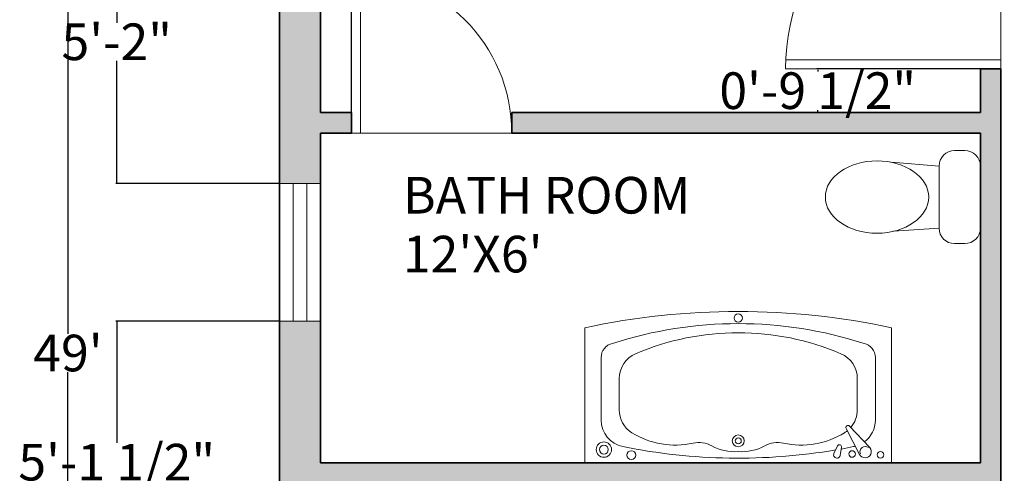
# Model space of a CAD drawing. Units: inches. Extents: x 638 to 1303, y 1 to 699.
# Tile 5 of 21: x 641 to 855, y 310 to 409. Entities that reach past the tile are written whole.
import ezdxf

# ---------------------------------------------------------------- set-up
doc = ezdxf.new("R2010")
doc.units = ezdxf.units.IN
doc.header["$MEASUREMENT"] = 0
for name, color, linetype, lineweight in [('A-ANNO-DIMS', 2, 'Continuous', 18), ('A-AREA-IDEN', 7, 'Continuous', 18), ('A-DOOR', 4, 'Continuous', 18), ('A-FLOR-FIXT', 9, 'Continuous', 18), ('A-GLAZ', 4, 'Continuous', 18), ('A-WALL', 7, 'Continuous', 35)]:
    doc.layers.add(name, color=color, linetype=linetype, lineweight=lineweight)
doc.layers.add('A-WALL-PATT', color=143, linetype='Continuous', lineweight=13, true_color=0x7aafdf)
doc.styles.get("Standard").update_dxf_attribs({"font": 'arial.ttf'})
doc.dimstyles.get("Standard").update_dxf_attribs({"dimtxt": 8, "dimasz": 0.18, "dimexe": 0.18, "dimexo": 0.0625, "dimgap": 0.09, "dimtad": 0, "dimtih": 1, "dimtoh": 1, "dimdec": 4, "dimzin": 0, "dimdsep": 46, "dimlunit": 3, "dimtxsty": 'Standard', "dimcen": 0.09, "dimadec": 0, "dimazin": 0, "dimtfac": 1, "dimtdec": 4, "dimtofl": 0, "dimtmove": 0, "dimatfit": 3, "dimfxl": 1, "dimtolj": 1, "dimtzin": 0, "dimarcsym": 0})

# ---------------------------------------------------------------- blocks, each defined once
blk = doc.blocks.new('*D1')
at = {"layer": 'A-ANNO-DIMS', "color": 0, "lineweight": -2, "transparency": 16777216}
for p, q in [((697.18, 629.82), (650.92, 629.82)), ((651.1, 629.64), (651.1, 339.99)), ((651.1, 42), (651.1, 331.64)), ((697.18, 41.82), (650.92, 41.82))]:
    blk.add_line(p, q, dxfattribs=at)
at = {"layer": 'A-ANNO-DIMS', "color": 0, "transparency": 16777216}
for points in [[(651.07, 629.64), (651.13, 629.64), (651.1, 629.82)], [(651.07, 42), (651.13, 42), (651.1, 41.82)]]:
    blk.add_solid(points, dxfattribs=at)
at = {"layer": 'Defpoints', "color": 0, "transparency": 16777216}
for p in [(697.24, 629.82), (651.1, 41.82), (697.24, 41.82)]:
    blk.add_point(p, dxfattribs=at)
at = {"layer": 'A-ANNO-DIMS', "color": 0, "transparency": 16777216, "insert": (651.1, 335.82), "char_height": 8, "attachment_point": 5}
blk.add_mtext("\\A1;49'", dxfattribs=at)
blk = doc.blocks.new('DOOR-SWING-35')
for p, q in [((33, 0), (33, 34.94)), ((35, 0), (35, 35)), ((0, 0), (35, 0))]:
    blk.add_line(p, q)
blk.add_arc((35, 0), 35, 90, 180)
blk = doc.blocks.new('WIN-30')
for p, q in [((30, 9), (0, 9)), ((0, 9), (0, 0)), ((30, 0), (30, 9)), ((0, 6), (30, 6)), ((0, 3), (30, 3)), ((0, 0), (30, 0))]:
    blk.add_line(p, q)
blk = doc.blocks.new('WC-CLOSE-COUPLED')
for p, q in [((28.2, 20.3), (30.45, 20.3)), ((24.81, 16.92), (14.41, 17.74)), ((24.81, 3.38), (24.81, 16.92)), ((33.84, 16.92), (33.84, 3.38)), ((24.81, 3.38), (14.9, 2.67)), ((30.45, 0), (28.2, 0))]:
    blk.add_line(p, q)
for centre, start, end in [((28.2, 16.92), 90, 180), ((30.45, 16.92), 0, 90), ((28.2, 3.38), 180, 270), ((30.45, 3.38), 270, 0)]:
    blk.add_arc(centre, 3.38, start, end)
blk.add_ellipse((11.28, 10.15), major_axis=(-11.28, 0), ratio=0.7)
blk = doc.blocks.new('*D57')
at = {"layer": 'A-ANNO-DIMS', "color": 0, "lineweight": -2, "transparency": 16777216}
for p, q in [((697.18, 342.79), (661.56, 342.79)), ((661.74, 342.61), (661.74, 316.23)), ((661.74, 281.4), (661.74, 307.78)), ((697.18, 281.22), (661.56, 281.22))]:
    blk.add_line(p, q, dxfattribs=at)
at = {"layer": 'A-ANNO-DIMS', "color": 0, "transparency": 16777216}
for points in [[(661.71, 342.61), (661.77, 342.61), (661.74, 342.79)], [(661.71, 281.4), (661.77, 281.4), (661.74, 281.22)]]:
    blk.add_solid(points, dxfattribs=at)
at = {"layer": 'Defpoints', "color": 0, "transparency": 16777216}
for p in [(661.74, 342.79), (697.24, 342.79), (697.24, 281.22)]:
    blk.add_point(p, dxfattribs=at)
at = {"layer": 'A-ANNO-DIMS', "color": 0, "transparency": 16777216, "insert": (661.74, 312), "char_height": 8, "attachment_point": 5}
blk.add_mtext('\\A1;5\'-1 1/2"', dxfattribs=at)
blk = doc.blocks.new('*D58')
at = {"layer": 'A-ANNO-DIMS', "color": 0, "lineweight": -2, "transparency": 16777216}
for p, q in [((697.18, 434.7), (661.56, 434.7)), ((661.74, 434.52), (661.74, 407.92)), ((661.74, 372.97), (661.74, 399.57)), ((697.18, 372.79), (661.56, 372.79))]:
    blk.add_line(p, q, dxfattribs=at)
at = {"layer": 'A-ANNO-DIMS', "color": 0, "transparency": 16777216}
for points in [[(661.71, 434.52), (661.77, 434.52), (661.74, 434.7)], [(661.71, 372.97), (661.77, 372.97), (661.74, 372.79)]]:
    blk.add_solid(points, dxfattribs=at)
at = {"layer": 'Defpoints', "color": 0, "transparency": 16777216}
for p in [(661.74, 434.7), (697.24, 434.7), (697.24, 372.79)]:
    blk.add_point(p, dxfattribs=at)
at = {"layer": 'A-ANNO-DIMS', "color": 0, "transparency": 16777216, "insert": (661.74, 403.75), "char_height": 8, "attachment_point": 5}
blk.add_mtext('\\A1;5\'-2"', dxfattribs=at)
blk = doc.blocks.new('*D66')
at = {"layer": 'A-ANNO-DIMS', "color": 0, "lineweight": -2, "transparency": 16777216}
for p, q in [((850.18, 397.83), (814.56, 397.83)), ((814.74, 397.65), (814.74, 397.3)), ((850.18, 388.32), (814.56, 388.32)), ((814.74, 388.5), (814.74, 388.85))]:
    blk.add_line(p, q, dxfattribs=at)
at = {"layer": 'A-ANNO-DIMS', "color": 0, "transparency": 16777216}
for points in [[(814.71, 397.65), (814.77, 397.65), (814.74, 397.83)], [(814.71, 388.5), (814.77, 388.5), (814.74, 388.32)]]:
    blk.add_solid(points, dxfattribs=at)
at = {"layer": 'Defpoints', "color": 0, "transparency": 16777216}
for p in [(814.74, 397.83), (850.24, 397.83), (850.24, 388.32)]:
    blk.add_point(p, dxfattribs=at)
at = {"layer": 'A-ANNO-DIMS', "color": 0, "transparency": 16777216, "insert": (814.74, 393.08), "char_height": 8, "attachment_point": 5}
blk.add_mtext('\\A1;0\'-9 1/2"', dxfattribs=at)
blk = doc.blocks.new('*D70')
at = {"layer": 'A-ANNO-DIMS', "color": 0, "lineweight": -2, "transparency": 16777216}
for p, q in [((706.24, 388.38), (706.24, 424)), ((706.42, 423.82), (712.77, 423.82)), ((712.95, 388.38), (712.95, 424)), ((712.95, 423.82), (713.13, 423.82))]:
    blk.add_line(p, q, dxfattribs=at)
at = {"layer": 'A-ANNO-DIMS', "color": 0, "transparency": 16777216}
for points in [[(706.42, 423.85), (706.42, 423.79), (706.24, 423.82)], [(712.77, 423.85), (712.77, 423.79), (712.95, 423.82)]]:
    blk.add_solid(points, dxfattribs=at)
at = {"layer": 'Defpoints', "color": 0, "transparency": 16777216}
for p in [(712.95, 423.82), (706.24, 388.32), (712.95, 388.32)]:
    blk.add_point(p, dxfattribs=at)
at = {"layer": 'A-ANNO-DIMS', "color": 0, "transparency": 16777216, "insert": (733.18, 423.82), "char_height": 8, "attachment_point": 5}
blk.add_mtext('\\A1;0\'-6 1/2"', dxfattribs=at)

msp = doc.modelspace()

# ---------------------------------------------------------------- hatches: boundary and pattern name
at = {"layer": 'A-WALL-PATT'}
h = msp.add_hatch(color=256, dxfattribs=at)
h.dxf.hatch_style = 1
h.paths.add_polyline_path([(973.34524, 629.81895), (793.35541, 629.81895), (793.35541, 620.81895), (850.23798, 620.81895), (922.23798, 620.81895), (922.23798, 524.81895), (908.94335, 524.81895), (908.94335, 520.31895), (926.73798, 520.31895), (926.73798, 544.31895), (979.3571, 544.31895), (979.3571, 548.81895), (926.73798, 548.81895), (926.73798, 620.81895), (973.34524, 620.81895)])
h.paths.add_polyline_path([(758.35541, 629.81895), (697.23798, 629.81895), (697.23798, 586.77451), (706.23798, 586.77451), (706.23798, 620.81895), (758.35541, 620.81895)])
h.paths.add_polyline_path([(1075.85281, 629.81895), (1003.34524, 629.81895), (1003.34524, 620.81895), (1046.73798, 620.81895), (1046.73798, 560.81895), (1046.73798, 548.81895), (1026.3571, 548.81895), (1026.3571, 544.31895), (1046.73798, 544.31895), (1046.73798, 486.87457), (1051.23798, 486.87457), (1051.23798, 556.31895), (1162.89753, 556.31895), (1162.89753, 560.81895), (1051.23798, 560.81895), (1051.23798, 620.81895), (1075.85281, 620.81895)])
h.paths.add_polyline_path([(1228.23798, 629.81895), (1105.85281, 629.81895), (1105.85281, 620.81895), (1219.23798, 620.81895), (1219.23798, 560.81895), (1197.89753, 560.81895), (1197.89753, 556.31895), (1219.23798, 556.31895), (1219.23798, 498.80084), (1228.23798, 498.80084)])
h.paths.add_polyline_path([(1051.23798, 439.87457), (1046.73798, 439.87457), (1046.73798, 407.81895), (1219.23798, 407.81895), (1219.23798, 381.66175), (1228.23798, 381.66175), (1228.23798, 451.80084), (1219.23798, 451.80084), (1219.23798, 412.31895), (1051.23798, 412.31895)])
h.paths.add_polyline_path([(1228.23798, 346.66175), (1219.23798, 346.66175), (1219.23798, 335.81895), (1046.73798, 335.81895), (1046.73798, 273.56895), (1051.23798, 273.56895), (1051.23798, 331.31895), (1219.23798, 331.31895), (1219.23798, 308.99654), (1228.23798, 308.99654)])
h.paths.add_polyline_path([(1228.23798, 261.99654), (1219.23798, 261.99654), (1219.23798, 211.31895), (1051.23798, 211.31895), (1051.23798, 226.56895), (1046.73798, 226.56895), (1046.73798, 211.31895), (983.84714, 211.31895), (983.84714, 206.81895), (1219.23798, 206.81895), (1219.23798, 166.83987), (1228.23798, 166.83987)])
h.paths.add_polyline_path([(1228.23798, 119.83987), (1219.23798, 119.83987), (1219.23798, 50.81895), (1197.89277, 50.81895), (1197.89277, 41.81895), (1228.23798, 41.81895)])
h.paths.add_polyline_path([(1162.89277, 50.81895), (1069.02949, 50.81895), (1069.02949, 41.81895), (1162.89277, 41.81895)])
h.paths.add_polyline_path([(1010.02949, 50.81895), (941.89631, 50.81895), (917.77455, 50.81895), (917.77455, 41.81895), (941.89631, 41.81895), (1010.02949, 41.81895)])
h.paths.add_polyline_path([(882.77455, 50.81895), (854.73798, 50.81895), (854.73798, 145.50379), (850.23798, 145.50379), (850.23798, 50.81895), (793.49755, 50.81895), (793.49755, 41.81895), (882.77455, 41.81895)])
h.paths.add_polyline_path([(746.49755, 50.81895), (706.23798, 50.81895), (706.23798, 96.57416), (697.23798, 96.57416), (697.23798, 41.81895), (746.49755, 41.81895)])
h.paths.add_polyline_path([(706.23798, 206.81895), (714.01165, 206.81895), (714.01165, 211.31895), (706.23798, 211.31895), (706.23798, 251.21966), (697.23798, 251.21966), (697.23798, 143.57416), (706.23798, 143.57416)])
h.paths.add_polyline_path([(923.84714, 211.31895), (854.73798, 211.31895), (854.73798, 397.8313), (850.23798, 397.8313), (850.23798, 388.31895), (747.9539, 388.31895), (747.9539, 383.81895), (850.23798, 383.81895), (850.23798, 311.81895), (706.23798, 311.81895), (706.23798, 342.78787), (697.23798, 342.78787), (697.23798, 281.21966), (706.23798, 281.21966), (706.23798, 307.31895), (850.23798, 307.31895), (850.23798, 211.31895), (749.01165, 211.31895), (749.01165, 206.81895), (850.23798, 206.81895), (850.23798, 192.50379), (854.73798, 192.50379), (854.73798, 206.81895), (923.84714, 206.81895)])
h.paths.add_polyline_path([(706.23798, 434.70471), (697.23798, 434.70471), (697.23798, 372.78787), (706.23798, 372.78787), (706.23798, 383.81895), (712.9539, 383.81895), (712.9539, 388.31895), (706.23798, 388.31895)])
h.paths.add_polyline_path([(706.23798, 520.31895), (850.23798, 520.31895), (850.23798, 444.8313), (854.73798, 444.8313), (854.73798, 520.31895), (861.94335, 520.31895), (861.94335, 524.81895), (706.23798, 524.81895), (706.23798, 551.77451), (697.23798, 551.77451), (697.23798, 481.70471), (706.23798, 481.70471)])

# ---------------------------------------------------------------- linework, layer by layer
at = {"layer": 'A-DOOR'}
for p, q in [((854.73798, 444.8313), (854.73798, 397.8313)), ((854.73798, 399.8313), (807.73798, 399.8313)), ((854.73798, 397.8313), (807.73798, 397.8313))]:
    msp.add_line(p, q, dxfattribs=at)
msp.add_arc((854.73798, 397.8313), 47, 90, 180, dxfattribs=at)
at = {"layer": 'A-FLOR-FIXT'}
for p, q in [((763.92818, 311.81895), (763.92818, 341.34645)), ((830.85718, 311.81895), (830.85718, 341.34645)), ((767.47148, 324.93057), (767.47148, 334.84331)), ((827.31388, 334.84331), (827.31388, 324.93057)), ((771.40848, 323.43888), (771.40848, 330.24465)), ((823.37688, 330.24465), (823.37688, 323.43888)), ((767.47148, 321.17536), (767.47148, 324.93057)), ((827.31388, 324.93057), (827.31388, 321.17536)), ((820.92178, 319.32097), (823.88637, 313.69568)), ((826.13748, 315.16947), (821.68251, 319.86636)), ((819.0491, 315.53177), (818.2862, 313.91052)), ((819.63657, 313.42497), (819.94253, 315.25261)), ((830.85718, 311.81895), (763.92818, 311.81895))]:
    msp.add_line(p, q, dxfattribs=at)
for centre, radius in [((797.39268, 343.45761), 0.90794), ((768.07127, 314.74254), 1.67445), ((797.39268, 316.65197), 1.29134), ((797.39268, 316.65197), 0.66142), ((768.07127, 314.74254), 0.96579), ((774.05145, 313.54509), 0.95683), ((822.2307, 313.78393), 0.71802), ((828.4314, 313.59179), 0.71802)]:
    msp.add_circle(centre, radius, dxfattribs=at)
for centre, radius, start, end in [((797.39268, 185.09129), 159.79846, 77.9118157, 102.0881843), ((797.39268, 252.99064), 89.2542, 72.0889709, 107.9110291), ((797.39268, 283.13689), 57.11385, 66.914883, 113.085117), ((770.62108, 334.84331), 3.1496, 102.424004, 180), ((824.16428, 334.84331), 3.1496, 0, 77.575996), ((777.31398, 330.24465), 5.9055, 113.085117, 180), ((817.47138, 330.24465), 5.9055, 0, 66.914883), ((777.31398, 323.43888), 5.9055, 180, 238.0738249), ((817.47138, 323.43888), 5.9055, 319.2863684, 0), ((773.37698, 321.17536), 5.9055, 180, 258.6168865), ((821.40838, 321.17536), 5.9055, 306.6595045, 0), ((783.66516, 333.63211), 17.91547, 238.0738249, 282.4290038), ((811.12019, 333.63211), 17.91547, 257.5709962, 301.9261751), ((817.47138, 323.43888), 5.9055, 301.9261751, 308.8465043), ((821.33973, 319.54124), 0.47244, 43.485816, 207.7897226), ((821.33973, 319.54124), 0.47244, 43.485816, 207.7897226), ((788.79214, 310.36942), 5.9055, 61.3911476, 102.4290038), ((805.99321, 310.36942), 5.9055, 77.5709962, 118.6088524), ((797.39268, 440.4614), 127.58505, 258.6168865, 279.5853712), ((796.57748, 324.64348), 10.35366, 241.3911476, 274.5158722), ((798.20787, 324.64348), 10.35366, 265.4841278, 298.6088524), ((818.93363, 313.59057), 0.72218, 153.702153, 346.7438582), ((819.47658, 315.33062), 0.47244, 350.4962776, 154.8001843), ((797.39268, 440.4614), 127.58505, 280.1511952, 281.3831135), ((821.40838, 321.17536), 5.9055, 281.3831135, 285.1221458), ((825.09615, 314.30392), 1.35408, 206.6916914, 39.7333965), ((825.11457, 314.27443), 1.15636, 52.6927353, 202.3523326)]:
    msp.add_arc(centre, radius, start, end, dxfattribs=at)
at = {"layer": 'A-WALL'}
for p, q in [((697.23798, 41.81895), (697.23798, 629.81895)), ((706.23798, 388.31895), (706.23798, 520.31895)), ((850.23798, 388.31895), (850.23798, 397.8313)), ((850.23798, 397.8313), (854.73798, 397.8313)), ((854.73798, 211.31895), (854.73798, 397.8313)), ((712.9539, 388.31895), (706.23798, 388.31895)), ((712.9539, 388.31895), (712.9539, 383.81895)), ((850.23798, 388.31895), (747.9539, 388.31895)), ((747.9539, 388.31895), (747.9539, 383.81895)), ((706.23798, 311.81895), (706.23798, 383.81895)), ((712.9539, 383.81895), (706.23798, 383.81895)), ((850.23798, 383.81895), (747.9539, 383.81895)), ((850.23798, 311.81895), (850.23798, 383.81895)), ((850.23798, 311.81895), (706.23798, 311.81895))]:
    msp.add_line(p, q, dxfattribs=at)

# ---------------------------------------------------------------- block references
at = {"layer": 'A-DOOR', "extrusion": (0, 0, -1), "zscale": -1}
msp.add_blockref('DOOR-SWING-35', (-747.95343, 383.819), dxfattribs=at)
at = {"layer": 'A-FLOR-FIXT'}
msp.add_blockref('WC-CLOSE-COUPLED', (816.40232, 359.7127), dxfattribs=at)
at = {"layer": 'A-GLAZ', "rotation": 269.9999999999995}
msp.add_blockref('WIN-30', (697.23803, 372.78768), dxfattribs=at)

# ---------------------------------------------------------------- texts
at = {"layer": 'A-AREA-IDEN'}
for s, p in [('BATH ROOM', (724.19157, 366.25979)), ("12'X6'", (724.19157, 353.4085))]:
    msp.add_text(s, height=8, dxfattribs=at).set_placement(p)

# ---------------------------------------------------------------- dimensions: what is measured, and where the dimension line sits
at = {"layer": 'A-ANNO-DIMS'}
for base, p1, p2, override, picture, middle in [((651.10111, 41.81895), (697.23798, 629.81895), (697.23798, 41.81895), {"dimclrd": 0, "dimclre": 0, "dimclrt": 0}, '*D1', (651.10111, 335.81895)), ((661.73798, 434.70471), (697.23798, 372.78787), (697.23798, 434.70471), {"dimdec": 1, "dimlfac": 1, "dimrnd": 0, "dimzin": 1, "dimdsep": 46, "dimlunit": 4, "dimfrac": 2}, '*D58', (661.73798, 403.74629)), ((814.73798, 397.8313), (850.23798, 388.31895), (850.23798, 397.8313), {"dimdec": 1, "dimlfac": 1, "dimrnd": 0, "dimzin": 1, "dimdsep": 46, "dimlunit": 4, "dimfrac": 2}, '*D66', (814.73798, 393.07513)), ((661.73798, 342.78787), (697.23798, 281.21966), (697.23798, 342.78787), {"dimdec": 1, "dimlfac": 1, "dimrnd": 0, "dimzin": 1, "dimdsep": 46, "dimlunit": 4, "dimfrac": 2}, '*D57', (661.73798, 312.00377))]:
    dim = msp.add_linear_dim(base=base, p1=p1, p2=p2, angle=90, dimstyle='Standard', override=override, dxfattribs=at)
    dim.commit()
    dim.dimension.update_dxf_attribs({"geometry": picture, "text_midpoint": middle})
dim = msp.add_linear_dim(base=(712.9539, 423.81895), p1=(706.23798, 388.31895), p2=(712.9539, 388.31895), dimstyle='Standard', override={"dimdec": 1, "dimlfac": 1, "dimrnd": 0, "dimzin": 1, "dimdsep": 46, "dimlunit": 4, "dimfrac": 2}, dxfattribs=at)
dim.commit()
dim.dimension.update_dxf_attribs({"geometry": '*D70', "text_midpoint": (733.17752, 423.81895)})

doc.saveas('drawing.dxf')
